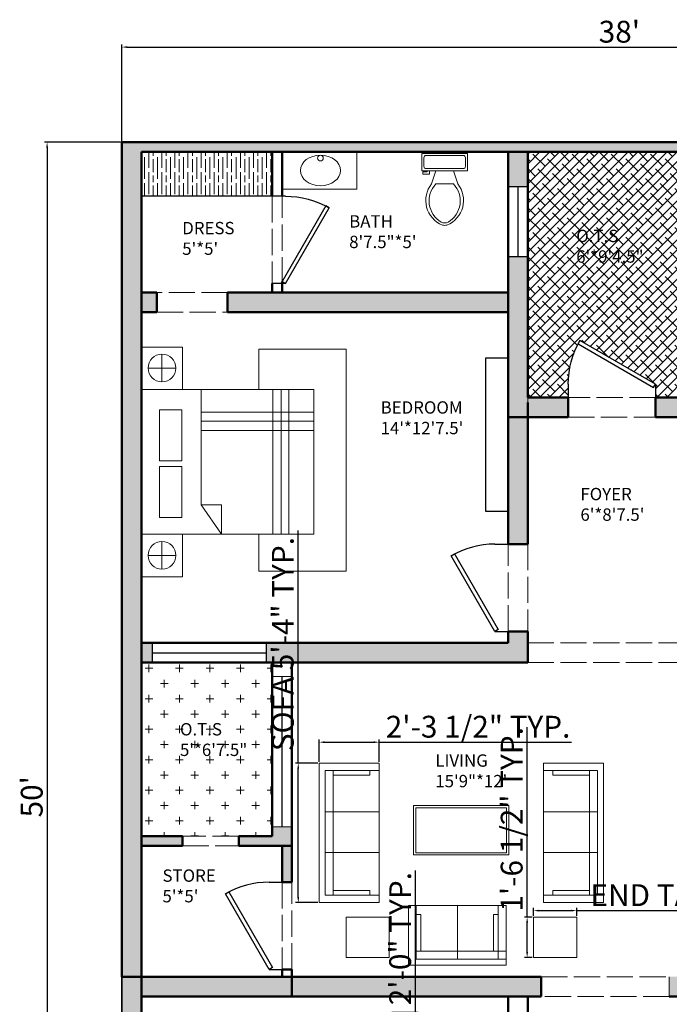
# Model space of a CAD drawing. Units: inches. Extents: x 2101 to 2698, y 3451 to 4160.
# Tile 2 of 3: x 2101 to 2399, y 3709 to 4160. Entities that reach past the tile are written whole.
import ezdxf

# ---------------------------------------------------------------- set-up
doc = ezdxf.new("R2010")
doc.units = ezdxf.units.IN
doc.linetypes.add('ACAD_ISO02W100', pattern=[15, 12, -3])
for name, color, linetype, lineweight in [('A-ANNO-DIMS', 40, 'Continuous', 18), ('A-AREA-IDEN', 40, 'Continuous', 18), ('A-FLOR-CASE', 132, 'Continuous', 25), ('A-FLOR-CASE-PATT', 132, 'Continuous', 13), ('A-FLOR-FIXT', 9, 'Continuous', 18), ('A-FLOR-PATT', 252, 'Continuous', 13), ('A-GLAZ-HIDN', 210, 'ACAD_ISO02W100', 18), ('A-WALL-OVHD', 150, 'ACAD_ISO02W100', 18), ('A-WALL-PATT', 150, 'Continuous', 13), ('C-PROP', 7, 'Continuous', 35), ('DOOR', 52, 'Continuous', 25), ('FURNITURE', 132, 'Continuous', 18), ('WALL', 150, 'Continuous', 50), ('WIN', 210, 'Continuous', 25)]:
    doc.layers.add(name, color=color, linetype=linetype, lineweight=lineweight)
doc.styles.get("Standard").update_dxf_attribs({"font": 'arial.ttf'})
doc.dimstyles.new('ISO-25', dxfattribs={"dimtxt": 10, "dimasz": 2.5, "dimexe": 1.25, "dimexo": 0.625, "dimtad": 1, "dimdec": 0, "dimlunit": 4, "dimtxsty": 'Standard', "dimcen": 2.5, "dimadec": 0, "dimazin": 0, "dimtfac": 1, "dimtdec": 0, "dimtmove": 0, "dimatfit": 3, "dimfxl": 1, "dimarcsym": 0})

# ---------------------------------------------------------------- blocks, each defined once
blk = doc.blocks.new('*U2')
for p, q in [((0, 0), (0, -6)), ((40, 0), (40, -6))]:
    blk.add_line(p, q)
blk.add_lwpolyline([(0, 0), (34.64, 20), (35.52, 18.48), (0.87, -1.52)], close=True)
blk.add_arc((0, 0), 40, 0, 30)
blk = doc.blocks.new('*U4')
for p, q in [((9.5, -6), (9.5, -2)), ((-10, -8.5), (-8, -8.5)), ((-10, -9.5), (-10, -8.5)), ((-8, -8.5), (-8, -8)), ((-7, -8), (-7, -9.5)), ((-4, -8), (-6, -14)), ((4, -8), (6, -14)), ((-7, -9.5), (-10, -9.5)), ((4, -14), (-4, -14))]:
    blk.add_line(p, q)
blk.add_lwpolyline([(10.5, -8), (10.5, 0), (-10.5, 0), (-10.5, -8)], close=True)
for points in [[(-9.5, -2), (-9.5, -6)], [(8.5, -1), (-8.5, -1)], [(-8.5, -7), (8.5, -7)]]:
    blk.add_lwpolyline(points)
for centre, radius, start, end in [((-8.62, -1.88), 0.884, 81.8699, 188.1301), ((8.62, -1.88), 0.884, 351.8699, 98.1301), ((-8.62, -6.12), 0.884, 171.8699, 278.1301), ((8.62, -6.12), 0.884, 261.8699, 8.1301), ((3.52, -21.58), 12.17, 141.4691, 247.9714), ((4.2, -21.82), 11.33, 136.3677, 238.9468), ((-3.52, -21.58), 12.17, 292.0284, 38.5307), ((-4.2, -21.82), 11.33, 301.053, 43.6321), ((0, -27.88), 4, 245.7318, 294.2682), ((0, -29), 4, 254.8605, 285.1395)]:
    blk.add_arc(centre, radius, start, end)
blk = doc.blocks.new('*D7')
at = {"layer": 'A-ANNO-DIMS', "color": 0, "lineweight": -2, "transparency": 16777216}
for p, q in [((2147.64, 4104.47), (2147.64, 4148.63)), ((2150.14, 4147.38), (2601.14, 4147.38)), ((2603.64, 4104.47), (2603.64, 4148.63))]:
    blk.add_line(p, q, dxfattribs=at)
at = {"layer": 'A-ANNO-DIMS', "color": 0, "lineweight": 100, "transparency": 16777216}
for points in [[(2150.14, 4147.8), (2150.14, 4146.97), (2147.64, 4147.38)], [(2601.14, 4147.8), (2601.14, 4146.97), (2603.64, 4147.38)]]:
    blk.add_solid(points, dxfattribs=at)
at = {"layer": 'Defpoints', "color": 0, "lineweight": 100, "transparency": 16777216}
for p in [(2603.64, 4147.38), (2147.64, 4103.85), (2603.64, 4103.85)]:
    blk.add_point(p, dxfattribs=at)
at = {"layer": 'A-ANNO-DIMS', "color": 0, "transparency": 16777216, "insert": (2375.64, 4153.12), "char_height": 10, "attachment_point": 5}
blk.add_mtext("38'", dxfattribs=at)
blk = doc.blocks.new('*D8')
at = {"layer": 'A-ANNO-DIMS', "color": 0, "lineweight": -2, "transparency": 16777216}
for p, q in [((2147.02, 4103.85), (2112.19, 4103.85)), ((2113.44, 4101.35), (2113.44, 3506.35)), ((2147.02, 3503.85), (2112.19, 3503.85))]:
    blk.add_line(p, q, dxfattribs=at)
at = {"layer": 'A-ANNO-DIMS', "color": 0, "lineweight": 100, "transparency": 16777216}
for points in [[(2113.03, 4101.35), (2113.86, 4101.35), (2113.44, 4103.85)], [(2113.03, 3506.35), (2113.86, 3506.35), (2113.44, 3503.85)]]:
    blk.add_solid(points, dxfattribs=at)
at = {"layer": 'Defpoints', "color": 0, "lineweight": 100, "transparency": 16777216}
for p in [(2147.64, 4103.85), (2113.44, 3503.85), (2147.64, 3503.85)]:
    blk.add_point(p, dxfattribs=at)
at = {"layer": 'A-ANNO-DIMS', "color": 0, "transparency": 16777216, "insert": (2107.71, 3803.85), "char_height": 10, "attachment_point": 5, "rotation": 90}
blk.add_mtext("50'", dxfattribs=at)
blk = doc.blocks.new('BED-DOUBLE-WITH-NIGHTSTANDS')
for p, q in [((9.75, 84.4), (9.75, 90.75)), ((9.75, 90.75), (9.75, 78.05)), ((95.59, 84.4), (95.59, 90.75)), ((95.59, 90.75), (95.59, 78.05)), ((16.1, 84.4), (3.4, 84.4)), ((9.75, 78.05), (9.75, 84.4)), ((9.75, 84.4), (16.1, 84.4)), ((101.95, 84.4), (89.24, 84.4)), ((95.59, 78.05), (95.59, 84.4)), ((95.59, 84.4), (101.95, 84.4)), ((19.5, 57.15), (32.87, 66.43)), ((85.75, 66.43), (32.87, 66.43)), ((32.87, 66.43), (32.87, 57.15)), ((66.97, 66.43), (66.97, 14.83)), ((71.27, 66.43), (71.27, 14.83)), ((75.39, 66.43), (75.39, 14.83)), ((32.87, 57.15), (19.5, 57.15)), ((19.5, 39.97), (2.47, 39.97)), ((2.47, 39.97), (2.47, 0)), ((104.25, 39.97), (85.75, 39.97)), ((104.25, 0), (104.25, 39.97)), ((85.75, 33.58), (19.5, 33.58)), ((85.75, 29.79), (19.5, 29.79)), ((85.75, 26.32), (19.5, 26.32)), ((2.47, 0), (104.25, 0))]:
    blk.add_line(p, q)
for points in [[(0, 93.85), (19.5, 93.85), (19.5, 74.95), (0, 74.95)], [(19.5, 93.85), (85.75, 93.85), (85.75, 14.83), (19.5, 14.83)], [(85.75, 93.85), (105.24, 93.85), (105.24, 74.95), (85.75, 74.95)], [(27.1, 85.6), (50.52, 85.6), (50.52, 75.29), (27.1, 75.29)], [(53.1, 85.6), (76.53, 85.6), (76.53, 75.29), (53.1, 75.29)]]:
    blk.add_lwpolyline(points, close=True)
for centre in [(9.75, 84.4), (95.59, 84.4)]:
    blk.add_circle(centre, 6.35)
blk = doc.blocks.new('SOFA-THREE-SEAT')
for p, q in [((27.45, 63.91), (0, 63.91)), ((0, 63.91), (0, 0)), ((27.45, 60.54), (27.45, 63.91)), ((6.46, 3.37), (6.46, 60.54)), ((23.21, 58.36), (23.21, 60.54)), ((6.46, 58.36), (6.46, 58.36)), ((6.46, 58.36), (23.21, 58.36)), ((27.45, 41.55), (2.74, 41.55)), ((27.45, 22.91), (2.74, 22.91)), ((6.46, 5.55), (23.21, 5.55)), ((23.21, 5.55), (23.21, 3.37)), ((27.45, 0), (27.45, 3.37)), ((0, 0), (27.45, 0))]:
    blk.add_line(p, q)
blk.add_lwpolyline([(2.74, 60.54), (27.45, 60.54), (27.45, 3.37), (2.74, 3.37)], close=True)
blk = doc.blocks.new('SIDE-TABLE')
blk.add_lwpolyline([(0, 18.49), (19.74, 18.49), (19.74, 0), (0, 0)], close=True)
blk = doc.blocks.new('*D22')
at = {"layer": 'A-ANNO-DIMS', "color": 0, "lineweight": -2, "transparency": 16777216}
for p, q in [((2282.24, 3705.14), (2282.24, 3770.01)), ((2271.34, 3705.14), (2283.49, 3705.14)), ((2282.24, 3683.69), (2282.24, 3702.64)), ((2271.34, 3681.19), (2283.49, 3681.19))]:
    blk.add_line(p, q, dxfattribs=at)
at = {"layer": 'A-ANNO-DIMS', "color": 0, "lineweight": 100, "transparency": 16777216}
for points in [[(2281.82, 3702.64), (2282.66, 3702.64), (2282.24, 3705.14)], [(2281.82, 3683.69), (2282.66, 3683.69), (2282.24, 3681.19)]]:
    blk.add_solid(points, dxfattribs=at)
at = {"layer": 'Defpoints', "color": 0, "lineweight": 100, "transparency": 16777216}
for p in [(2270.71, 3705.14), (2282.24, 3705.14), (2270.71, 3681.19)]:
    blk.add_point(p, dxfattribs=at)
at = {"layer": 'A-ANNO-DIMS', "color": 0, "transparency": 16777216, "insert": (2276.51, 3738.83), "char_height": 10, "attachment_point": 5, "rotation": 90}
blk.add_mtext('2\'-0" TYP.', dxfattribs=at)
blk = doc.blocks.new('*D23')
at = {"layer": 'A-ANNO-DIMS', "color": 0, "lineweight": -2, "transparency": 16777216}
for p, q in [((2228.53, 3819.27), (2228.53, 3925.84)), ((2237.49, 3819.27), (2227.28, 3819.27)), ((2228.53, 3757.85), (2228.53, 3816.77)), ((2237.49, 3755.35), (2227.28, 3755.35))]:
    blk.add_line(p, q, dxfattribs=at)
at = {"layer": 'A-ANNO-DIMS', "color": 0, "lineweight": 100, "transparency": 16777216}
for points in [[(2228.11, 3816.77), (2228.94, 3816.77), (2228.53, 3819.27)], [(2228.11, 3757.85), (2228.94, 3757.85), (2228.53, 3755.35)]]:
    blk.add_solid(points, dxfattribs=at)
at = {"layer": 'Defpoints', "color": 0, "lineweight": 100, "transparency": 16777216}
for p in [(2228.53, 3819.27), (2238.12, 3819.27), (2238.12, 3755.35)]:
    blk.add_point(p, dxfattribs=at)
at = {"layer": 'A-ANNO-DIMS', "color": 0, "transparency": 16777216, "insert": (2222.73, 3873.8), "char_height": 10, "attachment_point": 5, "rotation": 90}
blk.add_mtext('SOFA 5\'-4" TYP.', dxfattribs=at)
blk = doc.blocks.new('*D24')
at = {"layer": 'A-ANNO-DIMS', "color": 0, "lineweight": -2, "transparency": 16777216}
for p, q in [((2238.12, 3819.89), (2238.12, 3830.1)), ((2240.62, 3828.85), (2263.06, 3828.85)), ((2265.56, 3819.89), (2265.56, 3830.1)), ((2265.56, 3828.85), (2353.74, 3828.85))]:
    blk.add_line(p, q, dxfattribs=at)
at = {"layer": 'A-ANNO-DIMS', "color": 0, "lineweight": 100, "transparency": 16777216}
for points in [[(2240.62, 3829.27), (2240.62, 3828.44), (2238.12, 3828.85)], [(2263.06, 3829.27), (2263.06, 3828.44), (2265.56, 3828.85)]]:
    blk.add_solid(points, dxfattribs=at)
at = {"layer": 'Defpoints', "color": 0, "lineweight": 100, "transparency": 16777216}
for p in [(2265.56, 3828.85), (2238.12, 3819.27), (2265.56, 3819.27)]:
    blk.add_point(p, dxfattribs=at)
at = {"layer": 'A-ANNO-DIMS', "color": 0, "transparency": 16777216, "insert": (2310.9, 3834.65), "char_height": 10, "attachment_point": 5}
blk.add_mtext('2\'-3 1/2" TYP.', dxfattribs=at)
blk = doc.blocks.new('*D25')
at = {"layer": 'A-ANNO-DIMS', "color": 0, "lineweight": -2, "transparency": 16777216}
for p, q in [((2336.34, 3749.33), (2336.34, 3752.92)), ((2338.84, 3751.67), (2353.58, 3751.67)), ((2356.08, 3749.33), (2356.08, 3752.92)), ((2356.08, 3751.67), (2525.08, 3751.67))]:
    blk.add_line(p, q, dxfattribs=at)
at = {"layer": 'A-ANNO-DIMS', "color": 0, "lineweight": 100, "transparency": 16777216}
for points in [[(2338.84, 3752.09), (2338.84, 3751.25), (2336.34, 3751.67)], [(2353.58, 3752.09), (2353.58, 3751.25), (2356.08, 3751.67)]]:
    blk.add_solid(points, dxfattribs=at)
at = {"layer": 'Defpoints', "color": 0, "lineweight": 100, "transparency": 16777216}
for p in [(2356.08, 3751.67), (2336.34, 3748.71), (2356.08, 3748.71)]:
    blk.add_point(p, dxfattribs=at)
at = {"layer": 'A-ANNO-DIMS', "color": 0, "transparency": 16777216, "insert": (2441.83, 3757.46), "char_height": 10, "attachment_point": 5}
blk.add_mtext('END TABLE 1\'-7 1/2" TYP.', dxfattribs=at)
blk = doc.blocks.new('*D26')
at = {"layer": 'A-ANNO-DIMS', "color": 0, "lineweight": -2, "transparency": 16777216}
for p, q in [((2333.38, 3748.71), (2333.38, 3835.77)), ((2335.72, 3748.71), (2332.13, 3748.71)), ((2333.38, 3732.72), (2333.38, 3746.21)), ((2335.72, 3730.22), (2332.13, 3730.22))]:
    blk.add_line(p, q, dxfattribs=at)
at = {"layer": 'A-ANNO-DIMS', "color": 0, "lineweight": 100, "transparency": 16777216}
for points in [[(2332.96, 3746.21), (2333.8, 3746.21), (2333.38, 3748.71)], [(2332.96, 3732.72), (2333.8, 3732.72), (2333.38, 3730.22)]]:
    blk.add_solid(points, dxfattribs=at)
at = {"layer": 'Defpoints', "color": 0, "lineweight": 100, "transparency": 16777216}
for p in [(2333.38, 3748.71), (2336.34, 3748.71), (2336.34, 3730.22)]:
    blk.add_point(p, dxfattribs=at)
at = {"layer": 'A-ANNO-DIMS', "color": 0, "transparency": 16777216, "insert": (2327.59, 3793.49), "char_height": 10, "attachment_point": 5, "rotation": 90}
blk.add_mtext('1\'-6 1/2" TYP.', dxfattribs=at)

msp = doc.modelspace()

# ---------------------------------------------------------------- hatches: boundary and pattern name
at = {"layer": 'A-FLOR-CASE-PATT'}
h = msp.add_hatch(dxfattribs=at)
h.set_pattern_fill('GOST_WOOD', color=256)
h.paths.add_polyline_path([(2216.64, 4094.85), (2216.64, 4099.35), (2156.64, 4099.35), (2156.64, 4079.06), (2216.64, 4079.06)])
at = {"layer": 'A-FLOR-PATT'}
h = msp.add_hatch(dxfattribs=at)
h.set_pattern_fill('ANSI38', color=256)
h.paths.add_polyline_path([(2405.64, 4094.85), (2405.64, 4099.35), (2333.64, 4099.35), (2333.64, 4094.85), (2333.64, 4025.85), (2333.64, 3986.85), (2352.22, 3986.85), (2352.22, 3992.85, -0.120537), (2356.74, 4011.31), (2356.7, 4011.33), (2357.58, 4012.85), (2392.22, 3992.85), (2392.22, 3986.85), (2405.64, 3986.85)])
h = msp.add_hatch(dxfattribs=at)
h.set_pattern_fill('CROSS', color=256, scale=1.1)
h.paths.add_polyline_path([(2216.64, 3865.35), (2156.64, 3865.35), (2156.64, 3785.85), (2216.64, 3785.85)])
at = {"layer": 'A-WALL-PATT'}
h = msp.add_hatch(color=256, dxfattribs=at)
h.dxf.hatch_style = 1
h.paths.add_polyline_path([(2333.64, 4094.85), (2333.64, 4099.35), (2324.64, 4099.35), (2324.64, 4094.85), (2324.64, 4083.45), (2333.64, 4083.45)])
h.paths.add_polyline_path([(2405.64, 4103.85), (2156.64, 4103.85), (2156.64, 4099.35), (2405.64, 4099.35)])
h.paths.add_polyline_path([(2156.64, 4099.35), (2147.64, 4099.35), (2147.64, 3721.35), (2156.64, 3721.35)])
h = msp.add_hatch(color=256, dxfattribs=at)
h.dxf.hatch_style = 1
h.paths.add_polyline_path([(2156.64, 4103.85), (2147.64, 4103.85), (2147.64, 4099.35), (2156.64, 4099.35)])
h.paths.add_polyline_path([(2163.74, 4034.85), (2156.64, 4034.85), (2156.64, 4025.85), (2163.74, 4025.85)])
h.paths.add_polyline_path([(2333.64, 3874.35), (2333.64, 3879.64), (2324.64, 3879.64), (2324.64, 3874.35), (2213.91, 3874.35), (2213.91, 3865.35), (2333.64, 3865.35)])
h.paths.add_polyline_path([(2333.64, 3977.85), (2324.64, 3977.85), (2324.64, 3934.78), (2324.64, 3919.64), (2333.64, 3919.64)])
h.paths.add_polyline_path([(2161.58, 3874.35), (2156.64, 3874.35), (2156.64, 3865.35), (2161.58, 3865.35)])
h.paths.add_polyline_path([(2541.41, 3935.85), (2414.64, 3935.85), (2414.64, 3938.14), (2405.64, 3938.14), (2405.64, 3926.85), (2541.41, 3926.85)])
h.paths.add_polyline_path([(2594.64, 3935.85), (2581.41, 3935.85), (2581.41, 3926.85), (2594.64, 3926.85)])
h.paths.add_polyline_path([(2539.14, 3926.85), (2530.14, 3926.85), (2530.14, 3862.35), (2556.24, 3862.35), (2556.24, 3866.85), (2539.14, 3866.85)])
h.paths.add_polyline_path([(2599.14, 3866.85), (2594.64, 3866.85), (2578.65, 3866.85), (2578.65, 3862.35), (2594.64, 3862.35), (2599.14, 3862.35)])
h.paths.add_polyline_path([(2414.64, 3885.48), (2405.64, 3885.48), (2405.64, 3809.85), (2414.64, 3809.85), (2414.64, 3818.85), (2414.64, 3842.85)])
h.paths.add_polyline_path([(2530.14, 3818.85), (2414.64, 3818.85), (2414.64, 3809.85), (2450.64, 3809.85), (2530.14, 3809.85)])
h.paths.add_polyline_path([(2414.64, 3809.85), (2405.64, 3809.85), (2405.64, 3721.35), (2414.64, 3721.35), (2414.64, 3725.85)])
h.paths.add_polyline_path([(2603.64, 3814.35), (2599.14, 3814.35), (2594.64, 3814.35), (2594.64, 3559.35), (2603.64, 3559.35)])
h.paths.add_polyline_path([(2594.64, 3814.35), (2530.14, 3814.35), (2530.14, 3809.85), (2594.64, 3809.85)])
h = msp.add_hatch(color=256, dxfattribs=at)
h.dxf.hatch_style = 1
h.paths.add_polyline_path([(2333.64, 4031.79), (2333.64, 4051.21), (2324.64, 4051.21), (2324.64, 4034.85), (2324.64, 4031.79), (2324.64, 3977.85), (2333.64, 3977.85), (2333.64, 3984.47), (2333.64, 3986.85)])
h.paths.add_polyline_path([(2352.22, 3986.85), (2333.64, 3986.85), (2333.64, 3984.47), (2333.64, 3977.85), (2352.22, 3977.85)])
h.paths.add_polyline_path([(2405.64, 3986.85), (2392.22, 3986.85), (2392.22, 3977.85), (2405.64, 3977.85)])
h.paths.add_polyline_path([(2414.64, 3991.02), (2405.64, 3991.02), (2405.64, 3977.85), (2414.64, 3977.85)], flags=17)
h.paths.add_polyline_path([(2603.64, 4103.85), (2405.64, 4103.85), (2405.64, 4099.35), (2405.64, 4086.33), (2414.64, 4086.33), (2414.64, 4094.85), (2594.64, 4094.85), (2594.64, 3926.85), (2599.14, 3926.85), (2599.14, 3862.35), (2603.64, 3862.35)])
h.paths.add_polyline_path([(2324.64, 4031.79), (2324.64, 4034.85), (2213.11, 4034.85), (2196.16, 4034.85), (2196.16, 4025.85), (2221.14, 4025.85), (2324.64, 4025.85)])
h.paths.add_polyline_path([(2333.64, 4099.35), (2324.64, 4099.35), (2324.64, 4094.85), (2324.64, 4083.45), (2333.64, 4083.45), (2333.64, 4094.85)])
h = msp.add_hatch(color=256, dxfattribs=at)
h.dxf.hatch_style = 1
h.paths.add_polyline_path([(2324.64, 4031.79), (2324.64, 4034.85), (2213.11, 4034.85), (2196.16, 4034.85), (2196.16, 4025.85), (2221.14, 4025.85), (2324.64, 4025.85)])
h.paths.add_polyline_path([(2163.74, 4034.85), (2156.64, 4034.85), (2156.64, 4025.85), (2163.74, 4025.85)])
h.paths.add_polyline_path([(2333.64, 4094.85), (2333.64, 4099.35), (2324.64, 4099.35), (2324.64, 4094.85), (2324.64, 4083.45), (2333.64, 4083.45)])
h.paths.add_polyline_path([(2333.64, 4051.21), (2324.64, 4051.21), (2324.64, 4034.85), (2324.64, 4031.79), (2324.64, 4025.85), (2324.64, 3977.85), (2333.64, 3977.85), (2333.64, 3984.47), (2333.64, 3986.85), (2333.64, 4031.79)])
h.paths.add_polyline_path([(2333.64, 3977.85), (2324.64, 3977.85), (2324.64, 3934.78), (2324.64, 3919.64), (2333.64, 3919.64)])
h.paths.add_polyline_path([(2352.22, 3986.85), (2333.64, 3986.85), (2333.64, 3984.47), (2333.64, 3977.85), (2352.22, 3977.85)])
h.paths.add_polyline_path([(2405.64, 3986.85), (2392.22, 3986.85), (2392.22, 3977.85), (2405.64, 3977.85)])
h.paths.add_polyline_path([(2414.64, 3991.02), (2405.64, 3991.02), (2405.64, 3977.85), (2414.64, 3977.85)])
h.paths.add_polyline_path([(2161.58, 3874.35), (2156.64, 3874.35), (2156.64, 3865.35), (2161.58, 3865.35)])
h.paths.add_polyline_path([(2333.64, 3879.64), (2324.64, 3879.64), (2324.64, 3874.35), (2213.91, 3874.35), (2213.91, 3865.35), (2333.64, 3865.35)])
h = msp.add_hatch(color=256, dxfattribs=at)
h.dxf.hatch_style = 1
h.paths.add_polyline_path([(2333.64, 4031.79), (2333.64, 4051.21), (2324.64, 4051.21), (2324.64, 4034.85), (2324.64, 4031.79), (2324.64, 3977.85), (2333.64, 3977.85), (2333.64, 3984.47), (2333.64, 3986.85)])
h.paths.add_polyline_path([(2324.64, 4034.85), (2213.11, 4034.85), (2196.16, 4034.85), (2196.16, 4025.85), (2221.14, 4025.85), (2324.64, 4025.85), (2324.64, 4031.79)])
h.paths.add_polyline_path([(2352.22, 3986.85), (2333.64, 3986.85), (2333.64, 3984.47), (2333.64, 3977.85), (2352.22, 3977.85)])
h.paths.add_polyline_path([(2405.64, 3986.85), (2392.22, 3986.85), (2392.22, 3977.85), (2405.64, 3977.85)])
h.paths.add_polyline_path([(2414.64, 3991.02), (2405.64, 3991.02), (2405.64, 3977.85), (2414.64, 3977.85)])
h = msp.add_hatch(color=256, dxfattribs=at)
h.dxf.hatch_style = 1
h.paths.add_polyline_path([(2225.64, 3721.35), (2156.64, 3721.35), (2156.64, 3712.35), (2225.64, 3712.35)])
h.paths.add_polyline_path([(2339.85, 3721.35), (2333.64, 3721.35), (2225.64, 3721.35), (2225.64, 3712.35), (2324.64, 3712.35), (2339.85, 3712.35)])
h.paths.add_polyline_path([(2422.2, 3721.35), (2398.52, 3721.35), (2398.52, 3712.35), (2422.2, 3712.35)])
h.paths.add_polyline_path([(2414.64, 3809.85), (2405.64, 3809.85), (2405.64, 3721.35), (2414.64, 3721.35), (2414.64, 3725.85)])
h.paths.add_polyline_path([(2594.64, 3721.35), (2558.64, 3721.35), (2465.82, 3721.35), (2465.82, 3712.35), (2594.64, 3712.35)])
h.paths.add_polyline_path([(2530.14, 3818.85), (2414.64, 3818.85), (2414.64, 3809.85), (2530.14, 3809.85)])
h.paths.add_polyline_path([(2594.64, 3814.35), (2530.14, 3814.35), (2530.14, 3809.85), (2594.64, 3809.85)])
h = msp.add_hatch(color=256, dxfattribs=at)
h.dxf.hatch_style = 1
h.paths.add_polyline_path([(2228.64, 3568.35), (2200.53, 3568.35), (2200.53, 3563.85), (2228.64, 3563.85)])
h.paths.add_polyline_path([(2339.85, 3721.35), (2333.64, 3721.35), (2225.64, 3721.35), (2225.64, 3712.35), (2324.64, 3712.35), (2339.85, 3712.35)])
h.paths.add_polyline_path([(2225.64, 3721.35), (2156.64, 3721.35), (2156.64, 3712.35), (2225.64, 3712.35)])
h.paths.add_polyline_path([(2225.64, 3790), (2216.64, 3790), (2216.64, 3785.85), (2201.25, 3785.85), (2201.25, 3781.35), (2225.64, 3781.35)])
h.paths.add_polyline_path([(2225.64, 3781.35), (2221.14, 3781.35), (2221.14, 3764.71), (2225.64, 3764.71)])
h.paths.add_polyline_path([(2175.48, 3785.85), (2156.64, 3785.85), (2156.64, 3781.35), (2175.48, 3781.35)])
h.paths.add_polyline_path([(2414.64, 3809.85), (2405.64, 3809.85), (2405.64, 3721.35), (2414.64, 3721.35), (2414.64, 3725.85)])
h.paths.add_polyline_path([(2422.2, 3721.35), (2398.52, 3721.35), (2398.52, 3712.35), (2422.2, 3712.35)])
h = msp.add_hatch(color=256, dxfattribs=at)
h.dxf.hatch_style = 1
h.paths.add_polyline_path([(2175.48, 3785.85), (2156.64, 3785.85), (2156.64, 3781.35), (2175.48, 3781.35)])
h.paths.add_polyline_path([(2225.64, 3790), (2216.64, 3790), (2216.64, 3785.85), (2201.25, 3785.85), (2201.25, 3781.35), (2225.64, 3781.35)])
h.paths.add_polyline_path([(2225.64, 3781.35), (2221.14, 3781.35), (2221.14, 3764.71), (2225.64, 3764.71)])
h = msp.add_hatch(color=256, dxfattribs=at)
h.dxf.hatch_style = 1
h.paths.add_polyline_path([(2175.48, 3785.85), (2156.64, 3785.85), (2156.64, 3781.35), (2175.48, 3781.35)])
h.paths.add_polyline_path([(2225.64, 3790), (2216.64, 3790), (2216.64, 3785.85), (2201.25, 3785.85), (2201.25, 3781.35), (2225.64, 3781.35)])
h.paths.add_polyline_path([(2225.64, 3781.35), (2221.14, 3781.35), (2221.14, 3764.71), (2225.64, 3764.71)])
h = msp.add_hatch(color=256, dxfattribs=at)
h.dxf.hatch_style = 1
h.paths.add_polyline_path([(2247.32, 3568.35), (2228.64, 3568.35), (2228.64, 3559.35), (2228.64, 3512.85), (2237.64, 3512.85), (2237.64, 3559.35), (2247.32, 3559.35)], flags=17)
h.paths.add_polyline_path([(2228.64, 3568.35), (2200.53, 3568.35), (2200.53, 3563.85), (2228.64, 3563.85)], flags=17)
h.paths.add_polyline_path([(2333.64, 3569.5), (2333.64, 3571.5), (2324.64, 3571.5), (2324.64, 3568.35), (2316.02, 3568.35), (2316.02, 3559.35), (2333.64, 3559.35)])
h.paths.add_polyline_path([(2237.64, 3512.85), (2228.64, 3512.85), (2156.64, 3512.85), (2156.64, 3721.35), (2147.64, 3721.35), (2147.64, 3503.85), (2237.64, 3503.85)])
h.paths.add_polyline_path([(2237.64, 3559.35), (2247.32, 3559.35), (2247.32, 3568.35), (2228.64, 3568.35), (2228.64, 3563.85), (2228.64, 3559.35), (2228.64, 3512.85), (2237.64, 3512.85)], flags=17)

# ---------------------------------------------------------------- linework, layer by layer
at = {"layer": 'A-FLOR-CASE'}
msp.add_line((2216.64, 4079.06), (2156.64, 4079.06), dxfattribs=at)
msp.add_lwpolyline([(2324.64, 4004.82), (2314.31, 4004.82), (2314.31, 3934.78), (2324.64, 3934.78)], close=True, dxfattribs=at)
at = {"layer": 'A-FLOR-FIXT'}
msp.add_lwpolyline([(2221.14, 4099.35), (2255.34, 4099.35), (2255.34, 4082.33), (2221.14, 4082.33)], close=True, dxfattribs=at)
msp.add_circle((2238.7, 4096.53), 1.31, dxfattribs=at)
msp.add_ellipse((2238.7, 4090.83), major_axis=(9.18, 0), ratio=0.764313, dxfattribs=at)
at = {"layer": 'A-GLAZ-HIDN'}
msp.add_lwpolyline([(2216.64, 3790), (2225.64, 3790), (2225.64, 3858.96), (2216.64, 3858.96)], close=True, dxfattribs=at)
at = {"layer": 'A-WALL-OVHD'}
msp.add_line((2333.64, 3986.85), (2333.64, 3984.47), dxfattribs=at)
msp.add_lwpolyline([(2147.64, 4099.35), (2147.64, 4103.85), (2405.64, 4103.85), (2405.64, 4099.35), (2156.64, 4099.35)], dxfattribs=at)
for points in [[(2216.64, 4039.06), (2221.14, 4039.06), (2221.14, 4079.06), (2216.64, 4079.06)], [(2163.74, 4025.85), (2196.16, 4025.85), (2196.16, 4034.85), (2163.74, 4034.85)], [(2352.22, 3977.85), (2392.22, 3977.85), (2392.22, 3986.85), (2352.22, 3986.85)], [(2324.64, 3919.64), (2333.64, 3919.64), (2333.64, 3879.64), (2324.64, 3879.64)], [(2333.64, 3865.35), (2405.64, 3865.35), (2405.64, 3874.35), (2333.64, 3874.35)], [(2175.48, 3781.35), (2201.25, 3781.35), (2201.25, 3785.85), (2175.48, 3785.85)], [(2221.14, 3724.71), (2225.64, 3724.71), (2225.64, 3764.71), (2221.14, 3764.71)], [(2339.85, 3721.35), (2398.52, 3721.35), (2398.52, 3712.35), (2339.85, 3712.35)]]:
    msp.add_lwpolyline(points, close=True, dxfattribs=at)
at = {"layer": 'C-PROP'}
for p, q in [((2147.64, 4103.85), (2603.64, 4103.85)), ((2147.64, 3503.85), (2147.64, 4103.85))]:
    msp.add_line(p, q, dxfattribs=at)
at = {"layer": 'FURNITURE'}
for p, q in [((2282.48, 3754.09), (2279.1, 3754.09)), ((2279.1, 3754.09), (2279.1, 3726.65)), ((2301.46, 3754.09), (2301.46, 3729.39)), ((2320.11, 3754.09), (2320.11, 3729.39)), ((2323.84, 3726.65), (2323.84, 3754.09)), ((2284.66, 3749.86), (2282.48, 3749.86)), ((2284.66, 3733.1), (2284.66, 3749.86)), ((2317.93, 3733.1), (2317.93, 3749.86)), ((2317.93, 3749.86), (2320.11, 3749.86)), ((2323.84, 3733.1), (2282.48, 3733.1)), ((2284.66, 3733.1), (2284.66, 3733.1)), ((2279.1, 3726.65), (2323.84, 3726.65))]:
    msp.add_line(p, q, dxfattribs=at)
for points in [[(2281.36, 3799.8), (2324.93, 3799.8), (2324.93, 3777.18), (2281.36, 3777.18)], [(2282.36, 3798.8), (2323.93, 3798.8), (2323.93, 3778.18), (2282.36, 3778.18)]]:
    msp.add_lwpolyline(points, close=True, dxfattribs=at)
msp.add_lwpolyline([(2323.84, 3729.39), (2282.48, 3729.39), (2282.48, 3754.09), (2323.84, 3754.09)], dxfattribs=at)
at = {"layer": 'WALL'}
for p, q in [((2147.64, 4103.85), (2405.64, 4103.85)), ((2156.64, 4099.35), (2405.64, 4099.35)), ((2156.64, 3512.85), (2156.64, 4099.35)), ((2156.64, 4099.35), (2216.64, 4099.35)), ((2156.64, 4099.35), (2324.64, 4099.35)), ((2216.64, 4094.85), (2216.64, 4099.35)), ((2221.14, 4099.35), (2324.64, 4099.35)), ((2221.14, 4094.85), (2221.14, 4099.35)), ((2324.64, 4094.85), (2324.64, 4099.35)), ((2333.64, 4094.85), (2333.64, 4099.35)), ((2333.64, 4099.35), (2405.64, 4099.35)), ((2216.64, 4094.85), (2216.64, 4079.06)), ((2221.14, 4094.85), (2221.14, 4079.06)), ((2324.64, 4094.85), (2324.64, 4034.85)), ((2333.64, 4094.85), (2333.64, 4025.85)), ((2216.64, 4039.06), (2216.64, 4034.85)), ((2221.14, 4039.96), (2221.14, 4034.85)), ((2163.74, 4034.85), (2156.64, 4034.85)), ((2163.74, 4034.85), (2163.74, 4025.85)), ((2216.64, 4034.85), (2196.16, 4034.85)), ((2196.16, 4034.85), (2196.16, 4025.85)), ((2324.64, 4034.85), (2213.11, 4034.85)), ((2324.64, 4031.79), (2324.64, 4034.85)), ((2324.64, 3977.85), (2324.64, 4031.79)), ((2333.64, 3986.85), (2333.64, 4031.79)), ((2156.64, 4025.85), (2156.64, 3874.35)), ((2163.74, 4025.85), (2156.64, 4025.85)), ((2221.14, 4025.85), (2196.16, 4025.85)), ((2324.64, 4025.85), (2213.11, 4025.85)), ((2324.64, 3919.64), (2324.64, 3984.47)), ((2352.22, 3986.85), (2333.64, 3986.85)), ((2333.64, 3919.64), (2333.64, 3984.47)), ((2405.64, 3986.85), (2392.22, 3986.85)), ((2352.22, 3977.85), (2324.64, 3977.85)), ((2405.64, 3977.85), (2392.22, 3977.85)), ((2324.64, 3919.64), (2333.64, 3919.64)), ((2324.64, 3874.35), (2324.64, 3879.64)), ((2333.64, 3865.35), (2333.64, 3879.64)), ((2156.64, 3874.35), (2324.64, 3874.35)), ((2156.64, 3865.35), (2333.64, 3865.35)), ((2156.64, 3865.35), (2156.64, 3785.85)), ((2216.64, 3785.85), (2216.64, 3865.35)), ((2225.64, 3781.35), (2225.64, 3865.35)), ((2156.64, 3785.85), (2175.48, 3785.85)), ((2201.25, 3785.85), (2216.64, 3785.85)), ((2156.64, 3781.35), (2175.48, 3781.35)), ((2156.64, 3781.35), (2156.64, 3721.35)), ((2201.25, 3781.35), (2225.64, 3781.35)), ((2221.14, 3781.35), (2221.14, 3764.71)), ((2221.14, 3764.71), (2221.14, 3781.35)), ((2225.64, 3781.35), (2225.64, 3764.71)), ((2221.14, 3721.35), (2221.14, 3724.71)), ((2221.14, 3724.71), (2221.14, 3721.35)), ((2225.64, 3724.71), (2225.64, 3712.35)), ((2156.64, 3721.35), (2216.64, 3721.35)), ((2156.64, 3721.35), (2333.64, 3721.35)), ((2221.14, 3721.35), (2216.64, 3721.35)), ((2333.64, 3721.35), (2339.85, 3721.35)), ((2339.85, 3721.35), (2339.85, 3712.35)), ((2156.64, 3712.35), (2225.64, 3712.35)), ((2156.64, 3712.35), (2324.64, 3712.35)), ((2324.64, 3712.35), (2324.64, 3704.35)), ((2324.64, 3712.35), (2339.85, 3712.35)), ((2333.64, 3712.35), (2333.64, 3704.35)), ((2333.64, 3712.35), (2333.64, 3704.35)), ((2398.52, 3712.35), (2425.82, 3712.35))]:
    msp.add_line(p, q, dxfattribs=at)
for points in [[(2156.64, 4099.35), (2156.64, 3721.35), (2147.64, 3721.35), (2147.64, 4103.85), (2156.64, 4103.85)], [(2352.22, 3977.85), (2352.22, 3986.85)], [(2392.22, 3986.85), (2392.22, 3977.85)], [(2324.64, 3919.64), (2333.64, 3919.64)], [(2333.64, 3879.64), (2324.64, 3879.64)], [(2175.48, 3785.85), (2175.48, 3781.35)], [(2201.25, 3781.35), (2201.25, 3785.85)], [(2221.14, 3764.71), (2225.64, 3764.71)], [(2225.64, 3724.71), (2221.14, 3724.71)]]:
    msp.add_lwpolyline(points, dxfattribs=at)
at = {"layer": 'WIN'}
for p, q in [((2329.14, 4083.45), (2329.14, 4051.21)), ((2161.58, 3869.85), (2213.91, 3869.85)), ((2221.14, 3790), (2221.14, 3858.96))]:
    msp.add_line(p, q, dxfattribs=at)
for points in [[(2324.64, 4083.45), (2333.64, 4083.45), (2333.64, 4051.21), (2324.64, 4051.21)], [(2161.58, 3865.35), (2213.91, 3865.35), (2213.91, 3874.35), (2161.58, 3874.35)]]:
    msp.add_lwpolyline(points, close=True, dxfattribs=at)

# ---------------------------------------------------------------- block references
at = {"layer": 'A-FLOR-FIXT'}
msp.add_blockref('*U4', (2295.6, 4098.68), dxfattribs=at)
at = {"layer": 'DOOR', "xscale": -1, "rotation": 270}
msp.add_blockref('*U2', (2222.64, 4039.06), dxfattribs=at)
at = {"layer": 'DOOR', "xscale": -1}
msp.add_blockref('*U2', (2392.22, 3992.85), dxfattribs=at)
at = {"layer": 'DOOR', "rotation": 90}
for p in [(2318.64, 3879.64), (2215.14, 3724.71)]:
    msp.add_blockref('*U2', p, dxfattribs=at)
at = {"layer": 'FURNITURE', "rotation": 90.00000000000006}
msp.add_blockref('BED-DOUBLE-WITH-NIGHTSTANDS', (2250.49, 3904.7), dxfattribs=at)
at = {"layer": 'FURNITURE'}
for name, p in [('SOFA-THREE-SEAT', (2238.12, 3755.35)), ('SIDE-TABLE', (2250.45, 3730.22)), ('SIDE-TABLE', (2336.34, 3730.22))]:
    msp.add_blockref(name, p, dxfattribs=at)
at = {"layer": 'FURNITURE', "extrusion": (0, 0, -1), "zscale": -1}
msp.add_blockref('SOFA-THREE-SEAT', (-2368.38, 3755.35), dxfattribs=at)

# ---------------------------------------------------------------- texts
at = {"layer": 'A-AREA-IDEN', "attachment_point": 1}
for s, insert, char_height in [('BATH\\P8\'7.5"*5\'', (2251.86, 4070.35), 5.657), ("DRESS\\P5'*5'", (2175.37, 4067.26), 5.657), ('O.T.S\\P6\'*9\'4.5"', (2355.89, 4063.67), 5.657), ("BEDROOM\\P14'*12'7.5'", (2266.26, 3985.07), 5.6568), ("FOYER\\P6'*8'7.5'", (2357.79, 3945.39), 5.657), ('O.T.S\\P5\'*6\'7.5"', (2174.34, 3837.61), 5.657), ('LIVING\\P15\'9"*12\'', (2291.32, 3823.28), 5.657), ("STORE\\P5'*5'", (2166.32, 3770.55), 5.657)]:
    msp.add_mtext_dynamic_manual_height_columns(s, width=91.5864, gutter_width=28.28, heights=[0], dxfattribs=dict(at, insert=insert, char_height=char_height))

# ---------------------------------------------------------------- dimensions: what is measured, and where the dimension line sits
at = {"layer": 'A-ANNO-DIMS'}
dim = msp.add_linear_dim(base=(2603.64, 4147.38), p1=(2147.64, 4103.85), p2=(2603.64, 4103.85), dimstyle='ISO-25', override={"dimclrd": 0, "dimclre": 0, "dimclrt": 0}, dxfattribs=at)
dim.commit()
dim.dimension.update_dxf_attribs({"geometry": '*D7', "text_midpoint": (2375.64, 4153.12)})
dim = msp.add_linear_dim(base=(2113.44, 3503.85), p1=(2147.64, 4103.85), p2=(2147.64, 3503.85), angle=90, dimstyle='ISO-25', override={"dimclrd": 0, "dimclre": 0, "dimclrt": 0}, dxfattribs=at)
dim.commit()
dim.dimension.update_dxf_attribs({"geometry": '*D8', "text_midpoint": (2107.71, 3803.85)})
for base, p1, p2, text, picture, middle in [((2228.53, 3819.27), (2238.12, 3755.35), (2238.12, 3819.27), 'SOFA <> TYP.', '*D23', (2222.73, 3873.8)), ((2333.38, 3748.71), (2336.34, 3730.22), (2336.34, 3748.71), '<> TYP.', '*D26', (2327.59, 3793.49)), ((2282.241, 3705.1377), (2270.7131, 3681.1925), (2270.7131, 3705.1377), '<> TYP.', '*D22', (2276.5103, 3738.8255))]:
    dim = msp.add_linear_dim(base=base, p1=p1, p2=p2, angle=90, text=text, dimstyle='ISO-25', override={"dimdec": 1, "dimlfac": 1, "dimrnd": 0, "dimzin": 1, "dimdsep": 46, "dimlunit": 4, "dimfrac": 2}, dxfattribs=at)
    dim.commit()
    dim.dimension.update_dxf_attribs({"geometry": picture, "text_midpoint": middle})
for base, p1, p2, text, picture, middle in [((2265.56, 3828.85), (2238.12, 3819.27), (2265.56, 3819.27), '<> TYP.', '*D24', (2310.9, 3834.65)), ((2356.08, 3751.67), (2336.34, 3748.71), (2356.08, 3748.71), 'END TABLE <> TYP.', '*D25', (2441.83, 3757.46))]:
    dim = msp.add_linear_dim(base=base, p1=p1, p2=p2, text=text, dimstyle='ISO-25', override={"dimdec": 1, "dimlfac": 1, "dimrnd": 0, "dimzin": 1, "dimdsep": 46, "dimlunit": 4, "dimfrac": 2}, dxfattribs=at)
    dim.commit()
    dim.dimension.update_dxf_attribs({"geometry": picture, "text_midpoint": middle})

doc.saveas('drawing.dxf')
